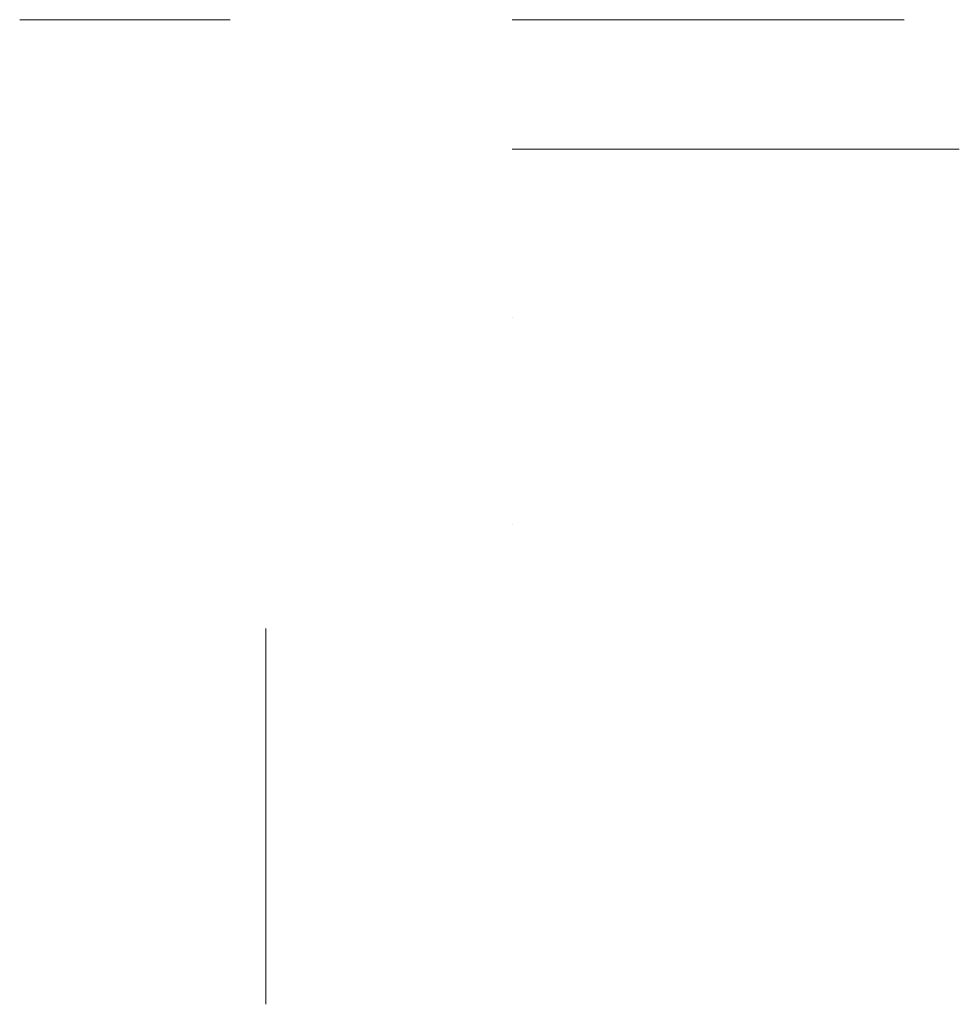
# Model space of a CAD drawing. Units: millimetres. Extents: x 91.9 to 164.4, y 479.8 to 555.8.
import ezdxf

# ---------------------------------------------------------------- set-up
doc = ezdxf.new("R2010")
doc.units = ezdxf.units.MM
doc.layers.add('M-CONS', color=8, linetype='Continuous', lineweight=13)

msp = doc.modelspace()

# ---------------------------------------------------------------- linework, layer by layer
at = {"layer": 'M-CONS'}
for p, q in [((91.911, 555.755, 64.179), (108.14, 555.755, -6.222)), ((129.911, 555.755, 64.179), (160.166, 555.755, 15.145)), ((129.911, 545.755, 64.179), (164.411, 545.755, 0.179)), ((129.911, 532.755, 96.179), (129.911, 532.755, 80.179)), ((129.911, 516.755, 80.179), (129.911, 516.755, 96.179)), ((110.911, 479.755, 83.179), (110.911, 508.755, 83.179)), ((110.911, 479.755, 83.179), (110.911, 508.755, 83.179))]:
    msp.add_line(p, q, dxfattribs=at)

doc.saveas('drawing.dxf')
